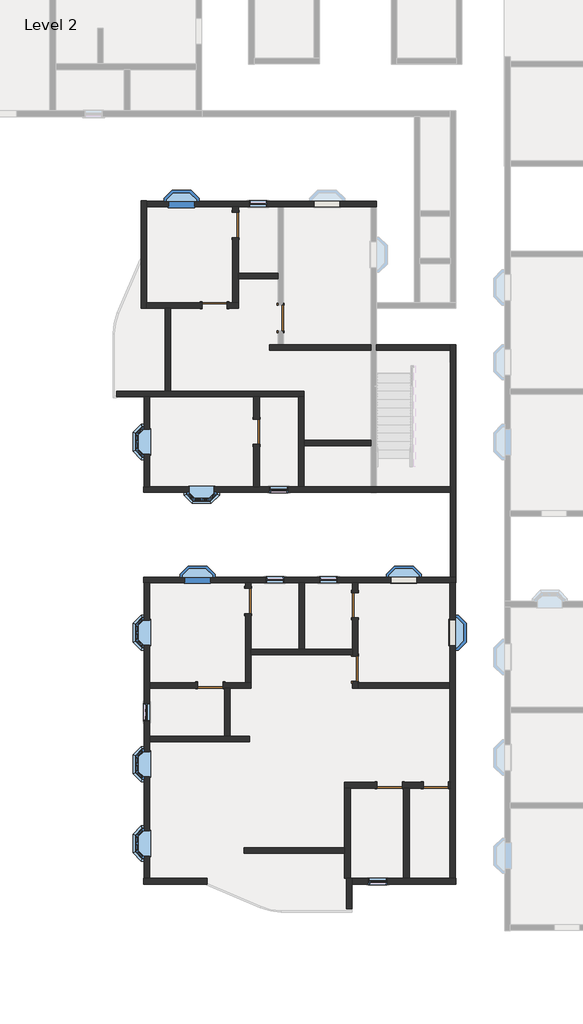
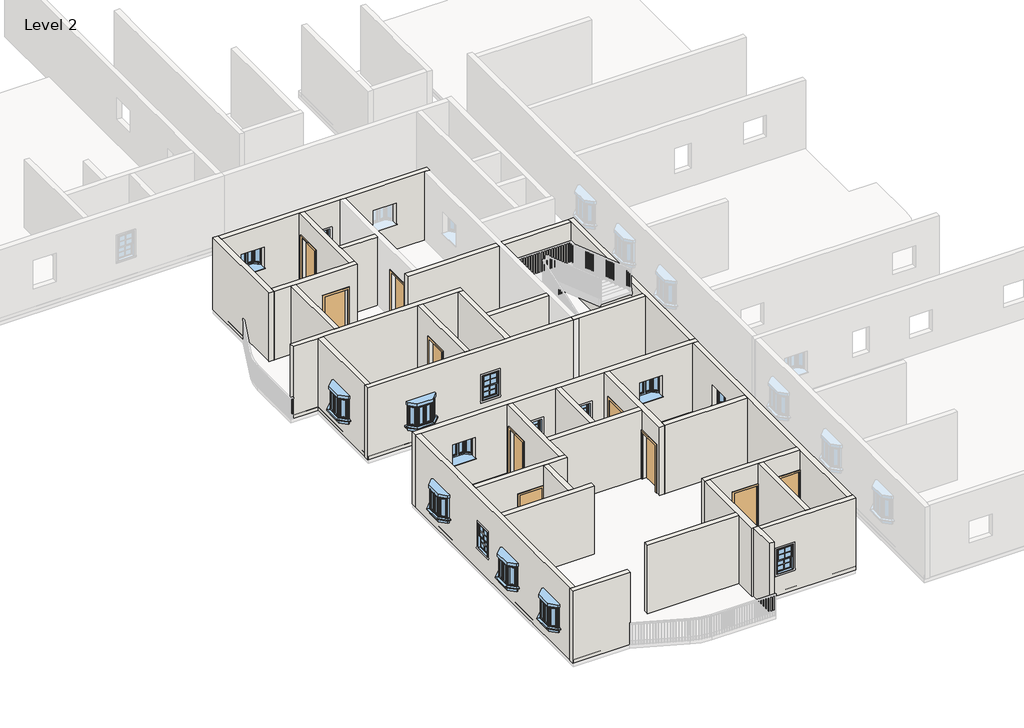
# One storey, part 1 of 14: 32 walls, 15 windows, 10 doors.
# Revit data of these elements (continued)
# Element 54 (IfcWindow, "Window-Double-Hung : 26\" x 42\"") (continued)
#   Window Inset = 0' - 0"
#   Interior Wall Closure = 0' - 1 1/2"
#   Frame Extension = 0' - 1 1/4"
#   Exterior Wall Closure = 0' - 0 1/2"
#   Interior Trim Visibility = yes
#   Indicator Visibility = yes
#   Exterior Trim Visibility = yes
#   Phase Created = New Construction
#   Materials on its faces: "Wood - Stained", "Glass", "Clad - White"
# Element 55 (IfcWindow, "Window-Double-Hung : 26\" x 42\"")
#   Mark = "107"
#   Window Inset = 0' - 0"
#   Interior Wall Closure = 0' - 1 1/2"
#   Frame Extension = 0' - 1 1/4"
#   Exterior Wall Closure = 0' - 0 1/2"
#   Interior Trim Visibility = yes
#   Indicator Visibility = yes
#   Exterior Trim Visibility = yes
#   Phase Created = New Construction
#   Materials on its faces: "Wood - Stained", "Glass", "Clad - White"
# Element 56 (IfcWindow, "Window-Double-Hung : 26\" x 42\"")
#   Mark = "108"
#   Window Inset = 0' - 0"
#   Interior Wall Closure = 0' - 1 1/2"
#   Frame Extension = 0' - 1 1/4"
#   Exterior Wall Closure = 0' - 0 1/2"
#   Interior Trim Visibility = yes
#   Indicator Visibility = yes
#   Exterior Trim Visibility = yes
#   Phase Created = New Construction
#   Materials on its faces: "Wood - Stained", "Glass", "Clad - White"
# Element 57 (IfcWindow, "Window-Double-Hung : 26\" x 42\"")
#   Mark = "109"
#   Window Inset = 0' - 0"
#   Interior Wall Closure = 0' - 1 1/2"
#   Frame Extension = 0' - 1 1/4"
#   Exterior Wall Closure = 0' - 0 1/2"
#   Interior Trim Visibility = yes
#   Indicator Visibility = yes
#   Exterior Trim Visibility = yes
#   Phase Created = New Construction
#   Materials on its faces: "Wood - Stained", "Glass", "Clad - White"
# Materials
#   "Door - Panel": class "Wood", colour RGB 210 159 95, transparency 0, Cost = 0
#   "Door - Frame": colour RGB 118 70 51, transparency 0, Cost = 0
#   "Window Frame": colour RGB 249 249 249, transparency 0
#   "Glass": class "Glass", colour RGB 0 128 192, transparency 0.75, Description = "Soda Lime Glass", Cost = 0
#   "Wood - Stained": class "Wood", colour RGB 224 178 126, transparency 0, Cost = 0
#   "Clad - White": class "Wood", colour RGB 242 242 238, transparency 0, Cost = 0
#   "Default Wall": colour RGB 128 128 128, transparency 0, Cost = 0
#   "Earth": class "Generic", colour RGB 97 75 62, transparency 0, Description = "Soil", Cost = 0
#   "Parking Stripe": class "Paint", colour RGB 250 250 91, transparency 0, Cost = 0
#   "Carpet (1)": class "Carpet", colour RGB 124 80 67, transparency 0, Description = "Interior finish", Cost = 0
#   "Softwood, Lumber": class "Wood", colour RGB 223 192 134, transparency 0, Description = "Pinus Echinata", Cost = 0
